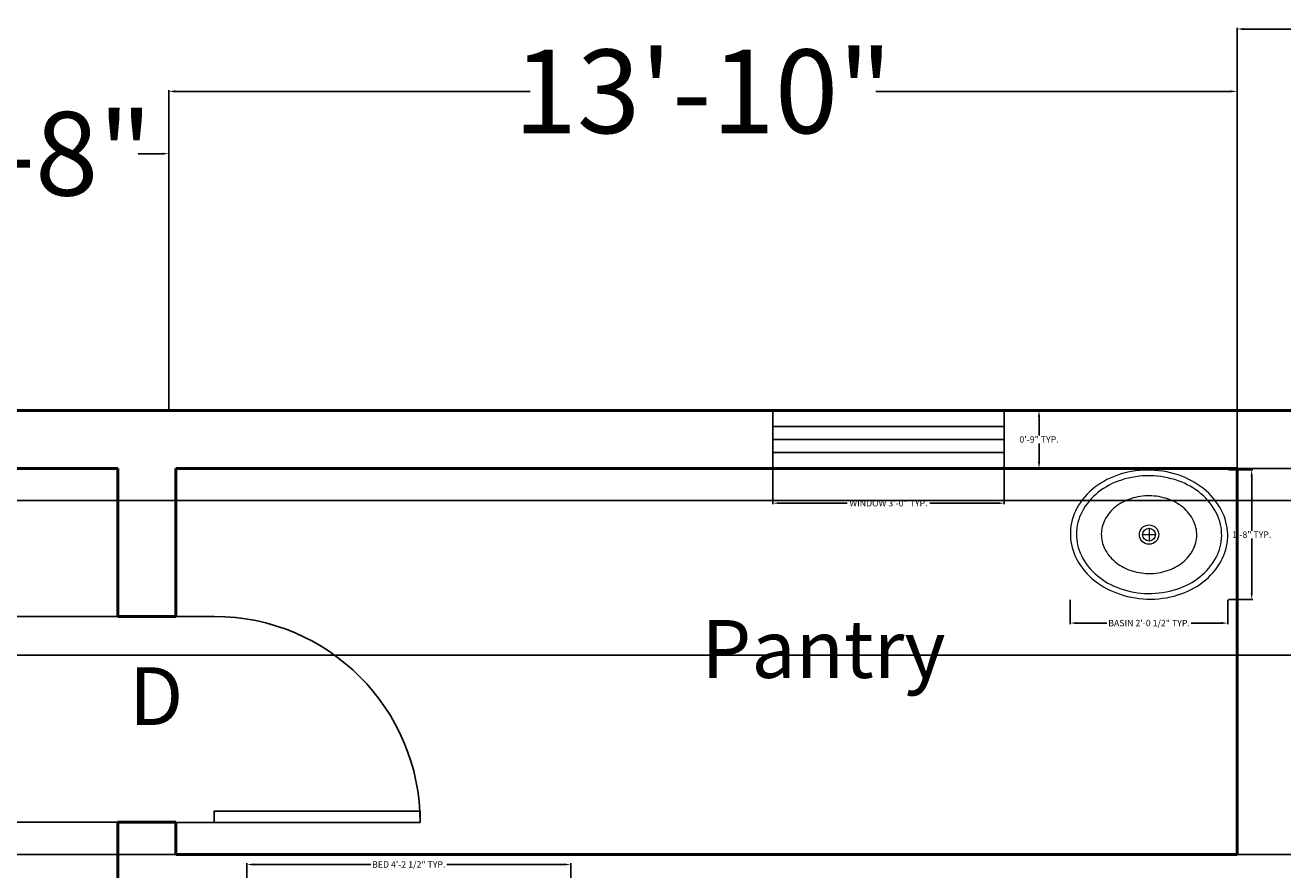
# Model space of a CAD drawing. Units: inches. Extents: x -364 to 705, y -52 to 1250.
# Tile 29 of 34: x 170 to 366, y 915 to 1046. Entities that reach past the tile are written whole.
import ezdxf

# ---------------------------------------------------------------- set-up
doc = ezdxf.new("R2010")
doc.units = ezdxf.units.IN
doc.header["$MEASUREMENT"] = 0
for name, color, linetype, lineweight in [('A-ANNO-DIMS', 4, 'Continuous', 18), ('A-ANNO-IDEN', 1, 'Continuous', 18), ('A-AREA-IDEN', 3, 'Continuous', 18), ('A-DOOR', 1, 'Continuous', 25), ('A-FLOR-FIXT', 9, 'Continuous', 18), ('A-GLAZ', 4, 'Continuous', 25), ('A-WALL', 41, 'Continuous', 50)]:
    doc.layers.add(name, color=color, linetype=linetype, lineweight=lineweight)
doc.styles.get("Standard").update_dxf_attribs({"font": 'arial.ttf'})
doc.dimstyles.get("Standard").update_dxf_attribs({"dimtxt": 1, "dimasz": 1, "dimexe": 0.18, "dimexo": 0.0625, "dimgap": 0.09, "dimtad": 0, "dimtih": 1, "dimtoh": 1, "dimdec": 0, "dimzin": 0, "dimdsep": 46, "dimlunit": 3, "dimtxsty": 'Standard', "dimcen": 0.09, "dimadec": 0, "dimazin": 0, "dimtfac": 1, "dimtdec": 0, "dimtofl": 0, "dimtmove": 0, "dimatfit": 3, "dimfxl": 1, "dimtolj": 1, "dimtzin": 0, "dimarcsym": 0})

# ---------------------------------------------------------------- blocks, each defined once
blk = doc.blocks.new('*U13')
for p, q in [((0, 0), (0, -6)), ((-32, 0), (-32, -6))]:
    blk.add_line(p, q)
blk.add_lwpolyline([(0, 0), (0, 32), (-1.75, 32), (-1.75, 0)], close=True)
blk.add_arc((0, 0), 32, 90, 180)
blk = doc.blocks.new('Sink - Oval top')
for p, q in [((-1, 0), (1, 0)), ((0, 1), (0, -1))]:
    blk.add_line(p, q)
for points in [[(-12.23, 0.39, 0.117634), (-11.46, -3.36, 0.104469), (-8.88, -6.8, 0.090016), (-5.08, -9.07, 0.08192), (-0.32, -10.02, 0.08192), (4.49, -9.38, 0.090016), (8.42, -7.36, 0.104469), (11.22, -4.09, 0.117634), (12.23, -0.39, 0.117634), (11.46, 3.36, 0.104469), (8.88, 6.8, 0.090016), (5.08, 9.07, 0.08192), (0.32, 10.02, 0.08192), (-4.49, 9.38, 0.090016), (-8.42, 7.36, 0.104469), (-11.22, 4.09, 0.117634)], [(-11.29, 0.16, 0.118622), (-10.52, -3.25, 0.104678), (-8.07, -6.36, 0.089562), (-4.54, -8.37, 0.081185), (-0.13, -9.15, 0.081185), (4.3, -8.49, 0.089562), (7.89, -6.58, 0.104678), (10.42, -3.55, 0.118622), (11.29, -0.16, 0.118622), (10.52, 3.25, 0.104678), (8.07, 6.36, 0.089562), (4.54, 8.37, 0.081185), (0.13, 9.15, 0.081185), (-4.3, 8.49, 0.089562), (-7.89, 6.58, 0.104678), (-10.42, 3.55, 0.118622)], [(-7.42, 0.08, 0.118283), (-6.91, -2.17, 0.104607), (-5.29, -4.21, 0.089718), (-2.97, -5.53, 0.081436), (-0.07, -6.04, 0.081436), (2.84, -5.59, 0.089718), (5.2, -4.33, 0.104607), (6.86, -2.32, 0.118283), (7.42, -0.08, 0.118283), (6.91, 2.17, 0.104607), (5.29, 4.21, 0.089718), (2.97, 5.53, 0.081436), (0.07, 6.04, 0.081436), (-2.84, 5.59, 0.089718), (-5.2, 4.33, 0.104607), (-6.86, 2.32, 0.118283)]]:
    blk.add_lwpolyline(points, format="xyb", close=True)
for radius in [1.5, 1]:
    blk.add_circle((0, 0), radius)
blk = doc.blocks.new('*D23')
at = {"layer": 'A-ANNO-DIMS', "color": 0, "lineweight": -2, "transparency": 16777216}
for p, q in [((28.58, 986.18), (28.58, 1127.53)), ((29.58, 1127.35), (265.4, 1127.35)), ((546.58, 1127.35), (310.76, 1127.35)), ((547.58, 986.18), (547.58, 1127.53))]:
    blk.add_line(p, q, dxfattribs=at)
at = {"layer": 'A-ANNO-DIMS', "color": 0, "transparency": 16777216}
for points in [[(29.58, 1127.52), (29.58, 1127.18), (28.58, 1127.35)], [(546.58, 1127.52), (546.58, 1127.18), (547.58, 1127.35)]]:
    blk.add_solid(points, dxfattribs=at)
at = {"layer": 'Defpoints', "color": 0, "transparency": 16777216}
for p in [(547.58, 1127.35), (28.58, 986.11), (547.58, 986.11)]:
    blk.add_point(p, dxfattribs=at)
at = {"layer": 'A-ANNO-DIMS', "color": 0, "transparency": 16777216, "insert": (288.08, 1127.35), "char_height": 1, "attachment_point": 5}
blk.add_mtext('\\A1;{\\H13x;43\'-3"}', dxfattribs=at)
blk = doc.blocks.new('*D25')
at = {"layer": 'A-ANNO-DIMS', "color": 0, "lineweight": -2, "transparency": 16777216}
for p, q in [((148.24, 986.18), (148.24, 1026.21)), ((149.24, 1026.03), (153.01, 1026.03)), ((191.5, 1026.03), (187.73, 1026.03)), ((192.5, 986.18), (192.5, 1026.21))]:
    blk.add_line(p, q, dxfattribs=at)
at = {"layer": 'A-ANNO-DIMS', "color": 0, "transparency": 16777216}
for points in [[(149.24, 1026.2), (149.24, 1025.86), (148.24, 1026.03)], [(191.5, 1026.2), (191.5, 1025.86), (192.5, 1026.03)]]:
    blk.add_solid(points, dxfattribs=at)
at = {"layer": 'Defpoints', "color": 0, "transparency": 16777216}
for p in [(192.5, 1026.03), (148.24, 986.11), (192.5, 986.11)]:
    blk.add_point(p, dxfattribs=at)
at = {"layer": 'A-ANNO-DIMS', "color": 0, "transparency": 16777216, "insert": (170.37, 1026.03), "char_height": 1, "attachment_point": 5}
blk.add_mtext('\\A1;{\\H13x;3\'-8"}', dxfattribs=at)
blk = doc.blocks.new('*D26')
at = {"layer": 'A-ANNO-DIMS', "color": 0, "lineweight": -2, "transparency": 16777216}
for p, q in [((192.5, 986.18), (192.5, 1035.9)), ((193.5, 1035.72), (248.68, 1035.72)), ((357.58, 1035.72), (302.4, 1035.72)), ((358.58, 977.18), (358.58, 1035.9))]:
    blk.add_line(p, q, dxfattribs=at)
at = {"layer": 'A-ANNO-DIMS', "color": 0, "transparency": 16777216}
for points in [[(193.5, 1035.88), (193.5, 1035.55), (192.5, 1035.72)], [(357.58, 1035.88), (357.58, 1035.55), (358.58, 1035.72)]]:
    blk.add_solid(points, dxfattribs=at)
at = {"layer": 'Defpoints', "color": 0, "transparency": 16777216}
for p in [(358.58, 1035.72), (192.5, 986.11), (358.58, 977.11)]:
    blk.add_point(p, dxfattribs=at)
at = {"layer": 'A-ANNO-DIMS', "color": 0, "transparency": 16777216, "insert": (275.54, 1035.72), "char_height": 1, "attachment_point": 5}
blk.add_mtext('\\A1;{\\H13x;13\'-10"}', dxfattribs=at)
blk = doc.blocks.new('*D27')
at = {"layer": 'A-ANNO-DIMS', "color": 0, "lineweight": -2, "transparency": 16777216}
for p, q in [((358.58, 986.18), (358.58, 1045.59)), ((359.58, 1045.41), (431.27, 1045.41)), ((546.58, 1045.41), (474.89, 1045.41)), ((547.58, 986.18), (547.58, 1045.59))]:
    blk.add_line(p, q, dxfattribs=at)
at = {"layer": 'A-ANNO-DIMS', "color": 0, "transparency": 16777216}
for points in [[(359.58, 1045.57), (359.58, 1045.24), (358.58, 1045.41)], [(546.58, 1045.57), (546.58, 1045.24), (547.58, 1045.41)]]:
    blk.add_solid(points, dxfattribs=at)
at = {"layer": 'Defpoints', "color": 0, "transparency": 16777216}
for p in [(547.58, 1045.41), (358.58, 986.11), (547.58, 986.11)]:
    blk.add_point(p, dxfattribs=at)
at = {"layer": 'A-ANNO-DIMS', "color": 0, "transparency": 16777216, "insert": (453.08, 1045.41), "char_height": 1, "attachment_point": 5}
blk.add_mtext('\\A1;{\\H13x;15\'-9"}', dxfattribs=at)
blk = doc.blocks.new('WIN-36-TRIPLE-LINE')
for p, q in [((36, 6.5), (0, 6.5)), ((36, 4.5), (0, 4.5)), ((36, 2.5), (0, 2.5))]:
    blk.add_line(p, q)
blk.add_lwpolyline([(36, 0), (0, 0), (0, 9), (36, 9)], close=True)
blk = doc.blocks.new('*D62')
at = {"layer": 'A-ANNO-DIMS', "color": 0, "lineweight": -2, "transparency": 16777216}
for p, q in [((204.64, 908.06), (204.64, 915.73)), ((205.64, 915.55), (223.9, 915.55)), ((253.99, 915.55), (235.72, 915.55)), ((254.99, 908.06), (254.99, 915.73))]:
    blk.add_line(p, q, dxfattribs=at)
at = {"layer": 'A-ANNO-DIMS', "color": 0, "transparency": 16777216}
for points in [[(205.64, 915.71), (205.64, 915.38), (204.64, 915.55)], [(253.99, 915.71), (253.99, 915.38), (254.99, 915.55)]]:
    blk.add_solid(points, dxfattribs=at)
at = {"layer": 'Defpoints', "color": 0, "transparency": 16777216}
for p in [(204.64, 915.55), (204.64, 907.99), (254.99, 907.99)]:
    blk.add_point(p, dxfattribs=at)
at = {"layer": 'A-ANNO-DIMS', "color": 0, "transparency": 16777216, "insert": (229.81, 915.55), "char_height": 1, "attachment_point": 5}
blk.add_mtext('\\A1;BED 4\'-2 1/2" TYP.', dxfattribs=at)
blk = doc.blocks.new('*D66')
at = {"layer": 'A-ANNO-DIMS', "color": 0, "lineweight": -2, "transparency": 16777216}
for p, q in [((332.61, 956.69), (332.61, 952.89)), ((357.16, 956.69), (357.16, 952.89)), ((333.61, 953.07), (338.32, 953.07)), ((356.16, 953.07), (351.46, 953.07))]:
    blk.add_line(p, q, dxfattribs=at)
at = {"layer": 'A-ANNO-DIMS', "color": 0, "transparency": 16777216}
for points in [[(333.61, 953.24), (333.61, 952.91), (332.61, 953.07)], [(356.16, 953.24), (356.16, 952.91), (357.16, 953.07)]]:
    blk.add_solid(points, dxfattribs=at)
at = {"layer": 'Defpoints', "color": 0, "transparency": 16777216}
for p in [(332.61, 956.75), (357.16, 956.75), (357.16, 953.07)]:
    blk.add_point(p, dxfattribs=at)
at = {"layer": 'A-ANNO-DIMS', "color": 0, "transparency": 16777216, "insert": (344.89, 953.07), "char_height": 1, "attachment_point": 5}
blk.add_mtext('\\A1;BASIN 2\'-0 1/2" TYP.', dxfattribs=at)
blk = doc.blocks.new('*D67')
at = {"layer": 'A-ANNO-DIMS', "color": 0, "lineweight": -2, "transparency": 16777216}
for p, q in [((357.23, 976.89), (361.03, 976.89)), ((360.85, 975.89), (360.85, 967.42)), ((360.85, 957.75), (360.85, 966.22)), ((357.23, 956.75), (361.03, 956.75))]:
    blk.add_line(p, q, dxfattribs=at)
at = {"layer": 'A-ANNO-DIMS', "color": 0, "transparency": 16777216}
for points in [[(360.68, 975.89), (361.01, 975.89), (360.85, 976.89)], [(360.68, 957.75), (361.01, 957.75), (360.85, 956.75)]]:
    blk.add_solid(points, dxfattribs=at)
at = {"layer": 'Defpoints', "color": 0, "transparency": 16777216}
for p in [(357.16, 976.89), (360.85, 976.89), (357.16, 956.75)]:
    blk.add_point(p, dxfattribs=at)
at = {"layer": 'A-ANNO-DIMS', "color": 0, "transparency": 16777216, "insert": (360.85, 966.82), "char_height": 1, "attachment_point": 5}
blk.add_mtext('\\A1;1\'-8" TYP.', dxfattribs=at)
blk = doc.blocks.new('*D70')
at = {"layer": 'A-ANNO-DIMS', "color": 0, "lineweight": -2, "transparency": 16777216}
for p, q in [((286.39, 977.05), (286.39, 971.53)), ((322.39, 977.05), (322.39, 971.53)), ((287.39, 971.71), (297.97, 971.71)), ((321.39, 971.71), (310.81, 971.71))]:
    blk.add_line(p, q, dxfattribs=at)
at = {"layer": 'A-ANNO-DIMS', "color": 0, "transparency": 16777216}
for points in [[(287.39, 971.88), (287.39, 971.55), (286.39, 971.71)], [(321.39, 971.88), (321.39, 971.55), (322.39, 971.71)]]:
    blk.add_solid(points, dxfattribs=at)
at = {"layer": 'Defpoints', "color": 0, "transparency": 16777216}
for p in [(286.39, 977.11), (322.39, 977.11), (322.39, 971.71)]:
    blk.add_point(p, dxfattribs=at)
at = {"layer": 'A-ANNO-DIMS', "color": 0, "transparency": 16777216, "insert": (304.39, 971.71), "char_height": 1, "attachment_point": 5}
blk.add_mtext('\\A1;WINDOW 3\'-0" TYP.', dxfattribs=at)
blk = doc.blocks.new('*D71')
at = {"layer": 'A-ANNO-DIMS', "color": 0, "lineweight": -2, "transparency": 16777216}
for p, q in [((322.45, 986.11), (327.97, 986.11)), ((327.79, 985.11), (327.79, 982.22)), ((327.79, 978.11), (327.79, 981.01)), ((322.45, 977.11), (327.97, 977.11))]:
    blk.add_line(p, q, dxfattribs=at)
at = {"layer": 'A-ANNO-DIMS', "color": 0, "transparency": 16777216}
for points in [[(327.62, 985.11), (327.96, 985.11), (327.79, 986.11)], [(327.62, 978.11), (327.96, 978.11), (327.79, 977.11)]]:
    blk.add_solid(points, dxfattribs=at)
at = {"layer": 'Defpoints', "color": 0, "transparency": 16777216}
for p in [(322.39, 986.11), (327.79, 986.11), (322.39, 977.11)]:
    blk.add_point(p, dxfattribs=at)
at = {"layer": 'A-ANNO-DIMS', "color": 0, "transparency": 16777216, "insert": (327.79, 981.61), "char_height": 1, "attachment_point": 5}
blk.add_mtext('\\A1;0\'-9" TYP.', dxfattribs=at)
blk = doc.blocks.new('*D95')
at = {"layer": 'A-ANNO-DIMS', "color": 0, "lineweight": -2, "transparency": 16777216}
for p, q in [((103.64, 972.11), (703.01, 972.11)), ((702.83, 971.11), (702.83, 960.72)), ((702.83, 949.11), (702.83, 959.51)), ((103.64, 948.11), (703.01, 948.11))]:
    blk.add_line(p, q, dxfattribs=at)
at = {"layer": 'A-ANNO-DIMS', "color": 0, "transparency": 16777216}
for points in [[(702.66, 971.11), (703, 971.11), (702.83, 972.11)], [(702.66, 949.11), (703, 949.11), (702.83, 948.11)]]:
    blk.add_solid(points, dxfattribs=at)
at = {"layer": 'Defpoints', "color": 0, "transparency": 16777216}
for p in [(103.58, 972.11), (702.83, 972.11), (103.58, 948.11)]:
    blk.add_point(p, dxfattribs=at)
at = {"layer": 'A-ANNO-DIMS', "color": 0, "transparency": 16777216, "insert": (702.83, 960.11), "char_height": 1, "attachment_point": 5}
blk.add_mtext('\\A1;2\'-0"', dxfattribs=at)
blk = doc.blocks.new('*D96')
at = {"layer": 'A-ANNO-DIMS', "color": 0, "lineweight": -2, "transparency": 16777216}
for p, q in [((358.64, 977.11), (703.01, 977.11)), ((702.83, 976.11), (702.83, 947.72)), ((702.83, 918.11), (702.83, 946.51)), ((358.64, 917.11), (703.01, 917.11))]:
    blk.add_line(p, q, dxfattribs=at)
at = {"layer": 'A-ANNO-DIMS', "color": 0, "transparency": 16777216}
for points in [[(702.66, 976.11), (703, 976.11), (702.83, 977.11)], [(702.66, 918.11), (703, 918.11), (702.83, 917.11)]]:
    blk.add_solid(points, dxfattribs=at)
at = {"layer": 'Defpoints', "color": 0, "transparency": 16777216}
for p in [(358.58, 977.11), (358.58, 917.11), (702.83, 917.11)]:
    blk.add_point(p, dxfattribs=at)
at = {"layer": 'A-ANNO-DIMS', "color": 0, "transparency": 16777216, "insert": (702.83, 947.11), "char_height": 1, "attachment_point": 5}
blk.add_mtext('\\A1;5\'-0"', dxfattribs=at)
blk = doc.blocks.new('*D103')
at = {"layer": 'A-ANNO-DIMS', "color": 0, "lineweight": -2, "transparency": 16777216}
for p, q in [((193.52, 954.1), (-126.85, 954.1)), ((-126.67, 953.1), (-126.67, 938.71)), ((-126.67, 923.11), (-126.67, 937.51)), ((193.52, 922.11), (-126.85, 922.11))]:
    blk.add_line(p, q, dxfattribs=at)
at = {"layer": 'A-ANNO-DIMS', "color": 0, "transparency": 16777216}
for points in [[(-126.84, 953.1), (-126.5, 953.1), (-126.67, 954.1)], [(-126.84, 923.11), (-126.5, 923.11), (-126.67, 922.11)]]:
    blk.add_solid(points, dxfattribs=at)
at = {"layer": 'Defpoints', "color": 0, "transparency": 16777216}
for p in [(-126.67, 954.1), (193.58, 954.1), (193.58, 922.11)]:
    blk.add_point(p, dxfattribs=at)
at = {"layer": 'A-ANNO-DIMS', "color": 0, "transparency": 16777216, "insert": (-126.67, 938.11), "char_height": 1, "attachment_point": 5}
blk.add_mtext('\\A1;2\'-8"', dxfattribs=at)
blk = doc.blocks.new('*D104')
at = {"layer": 'A-ANNO-DIMS', "color": 0, "lineweight": -2, "transparency": 16777216}
for p, q in [((193.52, 922.11), (-126.85, 922.11)), ((-126.67, 921.11), (-126.67, 920.22)), ((-126.67, 918.11), (-126.67, 919.01)), ((193.52, 917.11), (-126.85, 917.11))]:
    blk.add_line(p, q, dxfattribs=at)
at = {"layer": 'A-ANNO-DIMS', "color": 0, "transparency": 16777216}
for points in [[(-126.84, 921.11), (-126.5, 921.11), (-126.67, 922.11)], [(-126.84, 918.11), (-126.5, 918.11), (-126.67, 917.11)]]:
    blk.add_solid(points, dxfattribs=at)
at = {"layer": 'Defpoints', "color": 0, "transparency": 16777216}
for p in [(-126.67, 922.11), (193.58, 922.11), (193.58, 917.11)]:
    blk.add_point(p, dxfattribs=at)
at = {"layer": 'A-ANNO-DIMS', "color": 0, "transparency": 16777216, "insert": (-126.67, 919.61), "char_height": 1, "attachment_point": 5}
blk.add_mtext('\\A1;0\'-5"', dxfattribs=at)

msp = doc.modelspace()

# ---------------------------------------------------------------- linework, layer by layer
at = {"layer": 'A-WALL'}
for p, q in [((547.58, 986.11), (28.58, 986.11)), ((184.58, 977.11), (148.58, 977.11)), ((184.58, 954.1), (184.58, 977.11)), ((358.58, 977.11), (193.58, 977.11)), ((193.58, 954.1), (193.58, 977.11)), ((358.58, 917.11), (358.58, 977.11)), ((193.58, 954.1), (184.58, 954.1)), ((184.58, 822.11), (184.58, 922.11)), ((193.58, 922.11), (184.58, 922.11)), ((193.58, 917.11), (193.58, 922.11)), ((358.58, 917.11), (193.58, 917.11))]:
    msp.add_line(p, q, dxfattribs=at)

# ---------------------------------------------------------------- block references
at = {"layer": 'A-DOOR', "rotation": 270}
msp.add_blockref('*U13', (199.58, 922.1), dxfattribs=at)
at = {"layer": 'A-FLOR-FIXT'}
msp.add_blockref('Sink - Oval top', (344.89, 966.82), dxfattribs=at)
at = {"layer": 'A-GLAZ'}
msp.add_blockref('WIN-36-TRIPLE-LINE', (286.39, 977.11), dxfattribs=at)

# ---------------------------------------------------------------- texts
at = {"layer": 'A-ANNO-IDEN', "insert": (186.33, 946.21), "char_height": 9, "attachment_point": 1}
msp.add_mtext_dynamic_manual_height_columns('D', width=22.7519, gutter_width=1, heights=[0], dxfattribs=at)
at = {"layer": 'A-AREA-IDEN', "insert": (275.29, 953.55), "char_height": 9, "attachment_point": 1}
msp.add_mtext_dynamic_manual_height_columns('Pantry', width=59.8586, gutter_width=1, heights=[0], dxfattribs=at)

# ---------------------------------------------------------------- dimensions: what is measured, and where the dimension line sits
at = {"layer": 'A-ANNO-DIMS'}
for base, p1, p2, text, override, picture, middle in [((547.58, 1127.35), (28.58, 986.11), (547.58, 986.11), '{\\H13x;<>}', {"dimclrd": 0, "dimclre": 0, "dimclrt": 0}, '*D23', (288.08, 1127.35)), ((547.58, 1045.41), (358.58, 986.11), (547.58, 986.11), '{\\H13x;<>}', {"dimclrd": 0, "dimclre": 0, "dimclrt": 0}, '*D27', (453.08, 1045.41)), ((358.58, 1035.72), (192.5, 986.11), (358.58, 977.11), '{\\H13x;<>}', {"dimclrd": 0, "dimclre": 0, "dimclrt": 0}, '*D26', (275.54, 1035.72)), ((192.5, 1026.03), (148.24, 986.11), (192.5, 986.11), '{\\H13x;<>}', {"dimclrd": 0, "dimclre": 0, "dimclrt": 0}, '*D25', (170.37, 1026.03)), ((322.39, 971.71), (286.39, 977.11), (322.39, 977.11), 'WINDOW <> TYP.', {"dimdec": 1, "dimlfac": 1, "dimrnd": 0, "dimzin": 1, "dimdsep": 46, "dimlunit": 4, "dimfrac": 2}, '*D70', (304.39, 971.71)), ((357.1633, 953.0719), (332.6124, 956.7546), (357.1633, 956.7546), 'BASIN <> TYP.', {"dimdec": 1, "dimlfac": 1, "dimrnd": 0, "dimzin": 1, "dimdsep": 46, "dimlunit": 4, "dimfrac": 2}, '*D66', (344.8879, 953.0719))]:
    dim = msp.add_linear_dim(base=base, p1=p1, p2=p2, text=text, dimstyle='Standard', override=override, dxfattribs=at)
    dim.commit()
    dim.dimension.update_dxf_attribs({"geometry": picture, "text_midpoint": middle})
for base, p1, p2, angle, text, picture, middle in [((327.79, 986.11), (322.39, 977.11), (322.39, 986.11), 90, '<> TYP.', '*D71', (327.79, 981.61)), ((360.85, 976.89), (357.16, 956.75), (357.16, 976.89), 90, '<> TYP.', '*D67', (360.85, 966.82)), ((204.6375, 915.5467), (254.987, 907.9942), (204.6375, 907.9942), 180, 'BED <> TYP.', '*D62', (229.8123, 915.5467))]:
    dim = msp.add_linear_dim(base=base, p1=p1, p2=p2, angle=angle, text=text, dimstyle='Standard', override={"dimdec": 1, "dimlfac": 1, "dimrnd": 0, "dimzin": 1, "dimdsep": 46, "dimlunit": 4, "dimfrac": 2}, dxfattribs=at)
    dim.commit()
    dim.dimension.update_dxf_attribs({"geometry": picture, "text_midpoint": middle})
for base, p1, p2, picture, middle in [((702.83, 917.11), (358.58, 977.11), (358.58, 917.11), '*D96', (702.83, 947.11)), ((702.83, 972.11), (103.58, 948.11), (103.58, 972.11), '*D95', (702.83, 960.11)), ((-126.67, 954.1), (193.58, 922.11), (193.58, 954.1), '*D103', (-126.67, 938.11)), ((-126.67, 922.11), (193.58, 917.11), (193.58, 922.11), '*D104', (-126.67, 919.61))]:
    dim = msp.add_linear_dim(base=base, p1=p1, p2=p2, angle=90, dimstyle='Standard', override={"dimdec": 1, "dimlfac": 1, "dimrnd": 0, "dimzin": 1, "dimdsep": 46, "dimlunit": 4, "dimfrac": 2}, dxfattribs=at)
    dim.commit()
    dim.dimension.update_dxf_attribs({"geometry": picture, "text_midpoint": middle})

doc.saveas('drawing.dxf')
